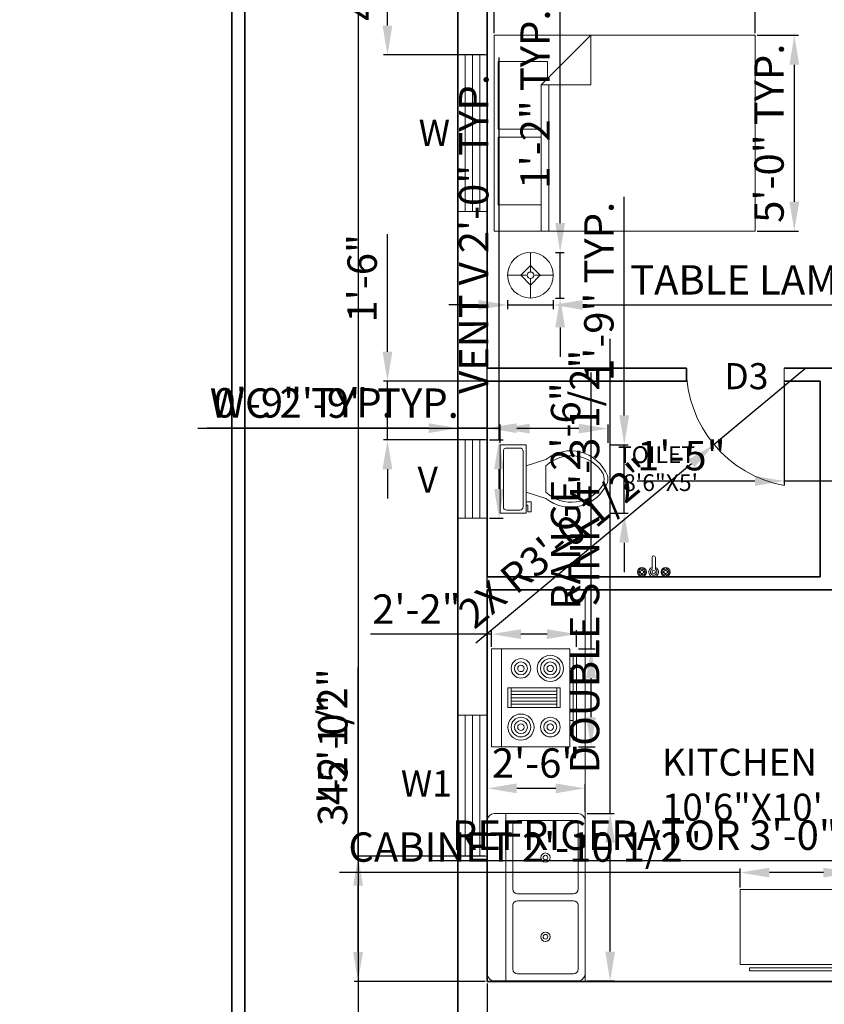
# Model space of a CAD drawing. Units: inches. Extents: x 2396 to 4051, y 1419 to 2191.
# Tile 2 of 7: x 2396 to 2642, y 1726 to 2028. Entities that reach past the tile are written whole.
import ezdxf

# ---------------------------------------------------------------- set-up
doc = ezdxf.new("R2010")
doc.units = ezdxf.units.IN
doc.layers.add('A-ANNO-TEXT', color=114, linetype='Continuous', lineweight=18, true_color=0x139b48)
doc.layers.add('A-GLAZ', color=52, linetype='Continuous', lineweight=18, true_color=0xc8c92d)
for name, color, linetype, lineweight in [('A-ANNO-TTLB', 7, 'Continuous', 35), ('A-AREA-IDEN', 6, 'Continuous', 18), ('A-DOOR', 4, 'Continuous', 18), ('A-EQPM', 8, 'Continuous', 18), ('A-FLOR-CASE', 9, 'Continuous', 18), ('A-FLOR-FIXT', 9, 'Continuous', 18), ('A-FURN', 8, 'Continuous', 18), ('A-WALL', 7, 'Continuous', 35), ('S-ANNO-DIMS', 2, 'Continuous', 18)]:
    doc.layers.add(name, color=color, linetype=linetype, lineweight=lineweight)
doc.styles.get("Standard").update_dxf_attribs({"font": 'arial.ttf'})
doc.dimstyles.new('ISO-25', dxfattribs={"dimtxt": 9, "dimasz": 9, "dimexe": 1.25, "dimexo": 0.625, "dimgap": 2, "dimtad": 1, "dimdec": 1, "dimlunit": 4, "dimtxsty": 'Standard', "dimcen": 2.5, "dimadec": 0, "dimazin": 0, "dimtfac": 1, "dimtdec": 1, "dimtmove": 0, "dimatfit": 3, "dimfxl": 1, "dimarcsym": 0})

# ---------------------------------------------------------------- blocks, each defined once
blk = doc.blocks.new('Wall Cabinet - 18 x 12 in side')
for points in [[(-12, -18), (-12, 0), (0, 0), (0, -18)], [(-13, -16.5), (-13, -1.5), (-12.5, -1.5), (-12.5, -16.5)]]:
    blk.add_lwpolyline(points, close=True)
blk = doc.blocks.new('Bed - Queen')
for p, q in [((0, -80.00003), (0, 0)), ((0, 0), (59.99999, 0)), ((59.99999, 0), (59.99999, -80.00003)), ((7.99999, -1.2), (28.79998, -1.2)), ((7.99999, -14.4), (7.99999, -1.2)), ((28.79998, -1.2), (28.79998, -14.4)), ((31.19999, -1.2), (51.99999, -1.2)), ((31.19999, -14.4), (31.19999, -1.2)), ((51.99999, -1.2), (51.99999, -16.4)), ((0, -14.4), (44.8, -14.4)), ((59.99999, -29.6), (44.8, -14.4)), ((44.8, -14.4), (44.8, -29.6)), ((44.8, -16.8), (0, -16.8)), ((51.99999, -16.4), (46.79936, -16.4)), ((44.8, -29.6), (59.99999, -29.6)), ((59.99999, -80.00003), (0, -80.00003))]:
    blk.add_line(p, q)
blk = doc.blocks.new('Lamp - Table')
for p, q in [((0, 7), (0, 1)), ((-1, 0), (-7, 0)), ((0, 3), (-3, 0)), ((-3, 0), (0, -3)), ((3, 0), (0, 3)), ((0, -3), (3, 0)), ((1, 0), (7, 0)), ((0, -1), (0, -7))]:
    blk.add_line(p, q)
for radius in [7, 1]:
    blk.add_circle((0, 0), radius)
blk = doc.blocks.new('Toilet - top')
for p, q in [((9.5, -6), (9.5, -2)), ((-10, -8.5), (-8, -8.5)), ((-10, -9.5), (-10, -8.5)), ((-8, -8.5), (-8, -8)), ((-7, -8), (-7, -9.5)), ((-4, -8), (-6, -14)), ((4, -8), (6, -14)), ((-7, -9.5), (-10, -9.5)), ((4, -14), (-4, -14))]:
    blk.add_line(p, q)
blk.add_lwpolyline([(10.5, -8), (10.5, 0), (-10.5, 0), (-10.5, -8)], close=True)
for points in [[(-9.5, -2), (-9.5, -6)], [(8.5, -1), (-8.5, -1)], [(-8.5, -7), (8.5, -7)]]:
    blk.add_lwpolyline(points)
for centre, radius, start, end in [((-8.62, -1.88), 0.884, 81.8699, 188.1301), ((8.62, -1.88), 0.884, 351.8699, 98.1301), ((-8.62, -6.12), 0.884, 171.8699, 278.1301), ((8.62, -6.12), 0.884, 261.8699, 8.1301), ((3.52, -21.58), 12.17, 141.4691, 247.9714), ((4.2, -21.82), 11.33, 136.3677, 238.9468), ((-3.52, -21.58), 12.17, 292.0284, 38.5307), ((-4.2, -21.82), 11.33, 301.053, 43.6321), ((0, -27.88), 4, 245.7318, 294.2682), ((0, -29), 4, 254.8605, 285.1395)]:
    blk.add_arc(centre, radius, start, end)
blk = doc.blocks.new('Faucet - Bathroom top')
for p, q in [((-4.107, 0.125), (-4.375, 0.125)), ((-3.75, 0.4788), (-3.75, 0.75)), ((-3.5, 0.482), (-3.5, 0.75)), ((-3.1461, 0.125), (-2.875, 0.125)), ((3.143, 0.125), (2.875, 0.125)), ((3.5, 0.4788), (3.5, 0.75)), ((3.75, 0.482), (3.75, 0.75)), ((4.1039, 0.125), (4.375, 0.125)), ((-4.1039, -0.125), (-4.375, -0.125)), ((-3.75, -0.4821), (-3.75, -0.75)), ((-3.5, -0.4789), (-3.5, -0.75)), ((-3.143, -0.125), (-2.875, -0.125)), ((-0.5, -0.8639), (-0.5, -4.5)), ((0.5, -4.5), (0.5, -0.8631)), ((3.1461, -0.125), (2.875, -0.125)), ((3.5, -0.4821), (3.5, -0.75)), ((3.75, -0.4789), (3.75, -0.75)), ((4.107, -0.125), (4.375, -0.125))]:
    blk.add_line(p, q)
for centre, radius in [((-3.625, 0), 1.375), ((-4.625, 0), 0.2795), ((-3.625, 0), 0.5), ((-3.625, 1), 0.2795), ((-2.625, 0), 0.2795), ((0, 0), 0.5), ((3.625, 0), 1.375), ((2.625, 0), 0.2795), ((3.625, 0), 0.5), ((3.625, 1), 0.2795), ((4.625, 0), 0.2795), ((-3.625, -1), 0.2795), ((3.625, -1), 0.2795)]:
    blk.add_circle(centre, radius)
for centre, radius, start, end in [((-3.625, 0), 1, 105.2407, 164.2093), ((-3.625, 0), 1, 16.44125, 74.07887), ((0, 0), 1.5, 289.6514, 250.3603), ((0, 0), 1, 300.3431, 239.7554), ((3.625, 0), 1, 106.12, 164.0884), ((3.625, 0), 1, 16.23422, 73.90469), ((-3.625, 0), 1, 196.2342, 253.9047), ((-3.625, 0), 1, 286.12, 344.0884), ((3.625, 0), 1, 196.4413, 254.0789), ((3.625, 0), 1, 285.2407, 344.2093), ((0, -4.5), 0.5, 180, 0)]:
    blk.add_arc(centre, radius, start, end)
blk = doc.blocks.new('Range-Oven - 30 in top')
for p, q in [((0, -3), (30, -3)), ((12, -6), (18, -6)), ((13, -20), (13, -6)), ((14, -6), (14, -20)), ((15, -20), (15, -6)), ((16, -6), (16, -20)), ((17, -20), (17, -6)), ((18, -20), (12, -20)), ((6, -24), (6, -25)), ((8, -25), (8, -24)), ((22, -25), (22, -24)), ((24, -24), (24, -25))]:
    blk.add_line(p, q)
for points in [[(0, -24), (0, 0), (30, 0), (30, -24)], [(12, -21), (12, -5), (18, -5), (18, -21)], [(2, -26), (2, -25), (28, -25), (28, -26)]]:
    blk.add_lwpolyline(points, close=True)
for centre, radius in [((6, -9), 4), ((6, -9), 3), ((24, -9), 3), ((6, -9), 2), ((6, -9), 1), ((24, -9), 2), ((24, -9), 1), ((6, -18), 3), ((24, -18), 4), ((24, -18), 3), ((6, -18), 2), ((6, -18), 1), ((24, -18), 2), ((24, -18), 1)]:
    blk.add_circle(centre, radius)
blk = doc.blocks.new('Sink-double - 36 in top')
for p, q in [((-18, -4), (18, -4)), ((-0.75, -18.5), (-0.75, -6.5)), ((0.75, -6.5), (0.75, -18.5))]:
    blk.add_line(p, q)
for points in [[(-16.5, 0), (16.5, 0)], [(-18, -19.5), (-18, -1.5)], [(18, -1.5), (18, -19.5)], [(-15.5, -5.5), (-1.75, -5.5)], [(1.75, -5.5), (15.5, -5.5)], [(-16.5, -18.5), (-16.5, -6.5)], [(16.5, -6.5), (16.5, -18.5)], [(16.5, -21), (-16.5, -21)], [(-1.75, -19.5), (-15.5, -19.5)], [(15.5, -19.5), (1.75, -19.5)]]:
    blk.add_lwpolyline(points)
for centre, radius in [((-8.5, -12.5), 1), ((-8.5, -12.5), 0.5), ((8.5, -12.5), 1), ((8.5, -12.5), 0.5)]:
    blk.add_circle(centre, radius)
for centre, radius, start, end in [((-16.5, -1.5), 1.5, 90, 180), ((16.5, -1.5), 1.5, 0, 90), ((-15.5, -6.5), 1, 90, 180), ((-1.75, -6.5), 1, 0, 90), ((1.75, -6.5), 1, 90, 180), ((15.5, -6.5), 1, 0, 90), ((-15.5, -18.5), 1, 180, 270), ((-1.75, -18.5), 1, 270, 0), ((1.75, -18.5), 1, 180, 270), ((15.5, -18.5), 1, 270, 0), ((-16.5, -19.5), 1.5, 180, 270), ((16.5, -19.5), 1.5, 270, 0)]:
    blk.add_arc(centre, radius, start, end)
blk = doc.blocks.new('WIN-W-48IN')
for p, q in [((0, 0), (0, 9)), ((0, 6.75), (48, 6.75)), ((48, 0), (48, 9)), ((0, 4.5), (48, 4.5)), ((0, 2.25), (48, 2.25))]:
    blk.add_line(p, q)
blk = doc.blocks.new('VENT-V-24IN')
for p, q in [((0, 0), (0, 9)), ((0, 6.75), (24, 6.75)), ((24, 0), (24, 9)), ((0, 4.5), (24, 4.5)), ((0, 2.25), (24, 2.25))]:
    blk.add_line(p, q)
blk = doc.blocks.new('WIN-W1-43P2IN')
for p, q in [((9, 43.2), (0, 43.2)), ((2.25, 0), (2.25, 43.2)), ((4.5, 0), (4.5, 43.2)), ((6.75, 0), (6.75, 43.2)), ((9, 0), (0, 0))]:
    blk.add_line(p, q)
blk = doc.blocks.new('DOOR-D3-36IN')
blk.add_line((30, 0), (30, 36))
blk.add_arc((36.6, 36), 36.6, 180, 259.6111)
blk = doc.blocks.new('*D40')
at = {"layer": 'Defpoints', "color": 0, "transparency": 16777216}
for p in [(2545.21, 1942.76), (2559.21, 1942.76), (2559.21, 1940.66)]:
    blk.add_point(p, dxfattribs=at)
at = {"layer": 'S-ANNO-DIMS', "color": 0, "lineweight": -2, "transparency": 16777216}
for p, q in [((2536.21, 1940.66), (2527.21, 1940.66)), ((2545.21, 1942.13), (2545.21, 1939.41)), ((2545.21, 1940.66), (2559.21, 1940.66)), ((2559.21, 1942.13), (2559.21, 1939.41)), ((2568.21, 1940.66), (2717.35, 1940.66))]:
    blk.add_line(p, q, dxfattribs=at)
at = {"layer": 'S-ANNO-DIMS', "color": 0, "transparency": 16777216}
for points in [[(2536.21, 1942.16), (2536.21, 1939.16), (2545.21, 1940.66)], [(2568.21, 1942.16), (2568.21, 1939.16), (2559.21, 1940.66)]]:
    blk.add_solid(points, dxfattribs=at)
at = {"layer": 'S-ANNO-DIMS', "color": 0, "transparency": 16777216, "insert": (2647.28, 1947.18), "char_height": 9, "attachment_point": 5}
blk.add_mtext('TABLE LAMP 1\'-2" TYP.', dxfattribs=at)
blk = doc.blocks.new('*D41')
at = {"layer": 'Defpoints', "color": 0, "transparency": 16777216}
for p in [(2559.21, 1956.76), (2561.31, 1956.76), (2559.21, 1942.76)]:
    blk.add_point(p, dxfattribs=at)
at = {"layer": 'S-ANNO-DIMS', "color": 0, "lineweight": -2, "transparency": 16777216}
for p, q in [((2561.31, 1965.76), (2561.31, 2032.77)), ((2559.83, 1956.76), (2562.56, 1956.76)), ((2561.31, 1942.76), (2561.31, 1956.76)), ((2559.83, 1942.76), (2562.56, 1942.76)), ((2561.31, 1933.76), (2561.31, 1924.76))]:
    blk.add_line(p, q, dxfattribs=at)
at = {"layer": 'S-ANNO-DIMS', "color": 0, "transparency": 16777216}
for points in [[(2559.81, 1965.76), (2562.81, 1965.76), (2561.31, 1956.76)], [(2559.81, 1933.76), (2562.81, 1933.76), (2561.31, 1942.76)]]:
    blk.add_solid(points, dxfattribs=at)
at = {"layer": 'S-ANNO-DIMS', "color": 0, "transparency": 16777216, "insert": (2554.79, 2003.76), "char_height": 9, "attachment_point": 5, "rotation": 90}
blk.add_mtext('1\'-2" TYP.', dxfattribs=at)
blk = doc.blocks.new('*D46')
at = {"layer": 'Defpoints', "color": 0, "transparency": 16777216}
for p in [(2541.07, 2035.3), (2541.07, 2023.3), (2621.07, 2023.3)]:
    blk.add_point(p, dxfattribs=at)
at = {"layer": 'S-ANNO-DIMS', "color": 0, "lineweight": -2, "transparency": 16777216}
for p, q in [((2541.07, 2035.3), (2395.68, 2035.3)), ((2541.07, 2023.93), (2541.07, 2036.55)), ((2612.07, 2035.3), (2550.07, 2035.3)), ((2621.07, 2023.93), (2621.07, 2036.55))]:
    blk.add_line(p, q, dxfattribs=at)
at = {"layer": 'S-ANNO-DIMS', "color": 0, "transparency": 16777216}
for points in [[(2550.07, 2036.8), (2550.07, 2033.8), (2541.07, 2035.3)], [(2612.07, 2036.8), (2612.07, 2033.8), (2621.07, 2035.3)]]:
    blk.add_solid(points, dxfattribs=at)
at = {"layer": 'S-ANNO-DIMS', "color": 0, "transparency": 16777216, "insert": (2463.87, 2042.23), "char_height": 9, "attachment_point": 5}
blk.add_mtext('QUEEN BED 6\'-8" TYP.', dxfattribs=at)
blk = doc.blocks.new('*D47')
at = {"layer": 'Defpoints', "color": 0, "transparency": 16777216}
for p in [(2621.07, 2023.3), (2633.07, 2023.3), (2621.07, 1963.3)]:
    blk.add_point(p, dxfattribs=at)
at = {"layer": 'S-ANNO-DIMS', "color": 0, "lineweight": -2, "transparency": 16777216}
for p, q in [((2621.7, 2023.3), (2634.32, 2023.3)), ((2633.07, 1972.3), (2633.07, 2014.3)), ((2621.7, 1963.3), (2634.32, 1963.3))]:
    blk.add_line(p, q, dxfattribs=at)
at = {"layer": 'S-ANNO-DIMS', "color": 0, "transparency": 16777216}
for points in [[(2631.57, 2014.3), (2634.57, 2014.3), (2633.07, 2023.3)], [(2631.57, 1972.3), (2634.57, 1972.3), (2633.07, 1963.3)]]:
    blk.add_solid(points, dxfattribs=at)
at = {"layer": 'S-ANNO-DIMS', "color": 0, "transparency": 16777216, "insert": (2626.48, 1993.3), "char_height": 9, "attachment_point": 5, "rotation": 90}
blk.add_mtext('5\'-0" TYP.', dxfattribs=at)
blk = doc.blocks.new('*D48')
at = {"layer": 'Defpoints', "color": 0, "transparency": 16777216}
for p in [(2542.93, 1902.76), (2542.93, 1897.8), (2575.98, 1897.8)]:
    blk.add_point(p, dxfattribs=at)
at = {"layer": 'S-ANNO-DIMS', "color": 0, "lineweight": -2, "transparency": 16777216}
for p, q in [((2542.93, 1902.76), (2450.26, 1902.76)), ((2542.93, 1898.43), (2542.93, 1904.01)), ((2566.98, 1902.76), (2551.93, 1902.76)), ((2575.98, 1898.43), (2575.98, 1904.01))]:
    blk.add_line(p, q, dxfattribs=at)
at = {"layer": 'S-ANNO-DIMS', "color": 0, "transparency": 16777216}
for points in [[(2551.93, 1904.26), (2551.93, 1901.26), (2542.93, 1902.76)], [(2566.98, 1904.26), (2566.98, 1901.26), (2575.98, 1902.76)]]:
    blk.add_solid(points, dxfattribs=at)
at = {"layer": 'S-ANNO-DIMS', "color": 0, "transparency": 16777216, "insert": (2492.1, 1909.41), "char_height": 9, "attachment_point": 5}
blk.add_mtext('WC 2\'-9" TYP.', dxfattribs=at)
blk = doc.blocks.new('*D49')
at = {"layer": 'Defpoints', "color": 0, "transparency": 16777216}
for p in [(2575.98, 1897.8), (2580.94, 1897.8), (2575.98, 1876.8)]:
    blk.add_point(p, dxfattribs=at)
at = {"layer": 'S-ANNO-DIMS', "color": 0, "lineweight": -2, "transparency": 16777216}
for p, q in [((2580.94, 1906.8), (2580.94, 1973.81)), ((2576.6, 1897.8), (2582.19, 1897.8)), ((2580.94, 1876.8), (2580.94, 1897.8)), ((2576.6, 1876.8), (2582.19, 1876.8)), ((2580.94, 1867.8), (2580.94, 1858.8))]:
    blk.add_line(p, q, dxfattribs=at)
at = {"layer": 'S-ANNO-DIMS', "color": 0, "transparency": 16777216}
for points in [[(2579.44, 1906.8), (2582.44, 1906.8), (2580.94, 1897.8)], [(2579.44, 1867.8), (2582.44, 1867.8), (2580.94, 1876.8)]]:
    blk.add_solid(points, dxfattribs=at)
at = {"layer": 'S-ANNO-DIMS', "color": 0, "transparency": 16777216, "insert": (2574.34, 1944.81), "char_height": 9, "attachment_point": 5, "rotation": 90}
blk.add_mtext('1\'-9" TYP.', dxfattribs=at)
blk = doc.blocks.new('*D52')
at = {"layer": 'Defpoints', "color": 0, "transparency": 16777216}
for p in [(2538.98, 1899.3), (2542.58, 1899.3), (2538.98, 1875.3)]:
    blk.add_point(p, dxfattribs=at)
at = {"layer": 'S-ANNO-DIMS', "color": 0, "lineweight": -2, "transparency": 16777216}
for p, q in [((2542.58, 1899.3), (2542.58, 2016.53)), ((2539.61, 1899.3), (2543.83, 1899.3)), ((2542.58, 1884.3), (2542.58, 1890.3)), ((2539.61, 1875.3), (2543.83, 1875.3))]:
    blk.add_line(p, q, dxfattribs=at)
at = {"layer": 'S-ANNO-DIMS', "color": 0, "transparency": 16777216}
for points in [[(2541.08, 1890.3), (2544.08, 1890.3), (2542.58, 1899.3)], [(2541.08, 1884.3), (2544.08, 1884.3), (2542.58, 1875.3)]]:
    blk.add_solid(points, dxfattribs=at)
at = {"layer": 'S-ANNO-DIMS', "color": 0, "transparency": 16777216, "insert": (2535.99, 1962.42), "char_height": 9, "attachment_point": 5, "rotation": 90}
blk.add_mtext('VENT V 2\'-0" TYP.', dxfattribs=at)
blk = doc.blocks.new('*D53')
at = {"layer": 'Defpoints', "color": 0, "transparency": 16777216}
for p in [(2529.98, 1902.9), (2529.98, 1899.3), (2538.98, 1899.3)]:
    blk.add_point(p, dxfattribs=at)
at = {"layer": 'S-ANNO-DIMS', "color": 0, "lineweight": -2, "transparency": 16777216}
for p, q in [((2520.98, 1902.9), (2453.12, 1902.9)), ((2529.98, 1899.93), (2529.98, 1904.15)), ((2538.98, 1902.9), (2529.98, 1902.9)), ((2538.98, 1899.93), (2538.98, 1904.15)), ((2547.98, 1902.9), (2556.98, 1902.9))]:
    blk.add_line(p, q, dxfattribs=at)
at = {"layer": 'S-ANNO-DIMS', "color": 0, "transparency": 16777216}
for points in [[(2520.98, 1904.4), (2520.98, 1901.4), (2529.98, 1902.9)], [(2547.98, 1904.4), (2547.98, 1901.4), (2538.98, 1902.9)]]:
    blk.add_solid(points, dxfattribs=at)
at = {"layer": 'S-ANNO-DIMS', "color": 0, "transparency": 16777216, "insert": (2482.55, 1909.5), "char_height": 9, "attachment_point": 5}
blk.add_mtext('0\'-9" TYP.', dxfattribs=at)
blk = doc.blocks.new('*D66')
at = {"layer": 'Defpoints', "color": 0, "transparency": 16777216}
for p in [(2661.68, 1770.32), (2661.68, 1764.92), (2697.68, 1764.92)]:
    blk.add_point(p, dxfattribs=at)
at = {"layer": 'S-ANNO-DIMS', "color": 0, "lineweight": -2, "transparency": 16777216}
for p, q in [((2661.68, 1765.55), (2661.68, 1771.57)), ((2697.68, 1765.55), (2697.68, 1771.57)), ((2661.68, 1770.32), (2521.84, 1770.32)), ((2688.68, 1770.32), (2670.68, 1770.32))]:
    blk.add_line(p, q, dxfattribs=at)
at = {"layer": 'S-ANNO-DIMS', "color": 0, "transparency": 16777216}
for points in [[(2670.68, 1771.82), (2670.68, 1768.82), (2661.68, 1770.32)], [(2688.68, 1771.82), (2688.68, 1768.82), (2697.68, 1770.32)]]:
    blk.add_solid(points, dxfattribs=at)
at = {"layer": 'S-ANNO-DIMS', "color": 0, "transparency": 16777216, "insert": (2587.26, 1776.98), "char_height": 9, "attachment_point": 5}
blk.add_mtext('REFRIGERATOR 3\'-0"', dxfattribs=at)
blk = doc.blocks.new('*D68')
at = {"layer": 'Defpoints', "color": 0, "transparency": 16777216}
for p in [(2616.45, 1766.68), (2616.45, 1761.5), (2650.99, 1761.5)]:
    blk.add_point(p, dxfattribs=at)
at = {"layer": 'S-ANNO-DIMS', "color": 0, "lineweight": -2, "transparency": 16777216}
for p, q in [((2616.45, 1766.68), (2493.68, 1766.68)), ((2616.45, 1762.12), (2616.45, 1767.93)), ((2641.99, 1766.68), (2625.45, 1766.68)), ((2650.99, 1762.12), (2650.99, 1767.93))]:
    blk.add_line(p, q, dxfattribs=at)
at = {"layer": 'S-ANNO-DIMS', "color": 0, "transparency": 16777216}
for points in [[(2625.45, 1768.18), (2625.45, 1765.18), (2616.45, 1766.68)], [(2641.99, 1768.18), (2641.99, 1765.18), (2650.99, 1766.68)]]:
    blk.add_solid(points, dxfattribs=at)
at = {"layer": 'S-ANNO-DIMS', "color": 0, "transparency": 16777216, "insert": (2550.56, 1773.33), "char_height": 9, "attachment_point": 5}
blk.add_mtext('CABINET 2\'-10 1/2"', dxfattribs=at)
blk = doc.blocks.new('*D72')
at = {"layer": 'Defpoints', "color": 0, "transparency": 16777216}
for p in [(2566.29, 1835.27), (2570.79, 1835.27), (2566.29, 1805.27)]:
    blk.add_point(p, dxfattribs=at)
at = {"layer": 'S-ANNO-DIMS', "color": 0, "lineweight": -2, "transparency": 16777216}
for p, q in [((2570.79, 1835.27), (2570.79, 1919.93)), ((2566.91, 1835.27), (2572.04, 1835.27)), ((2570.79, 1814.27), (2570.79, 1826.27)), ((2566.91, 1805.27), (2572.04, 1805.27))]:
    blk.add_line(p, q, dxfattribs=at)
at = {"layer": 'S-ANNO-DIMS', "color": 0, "transparency": 16777216}
for points in [[(2569.29, 1826.27), (2572.29, 1826.27), (2570.79, 1835.27)], [(2569.29, 1814.27), (2572.29, 1814.27), (2570.79, 1805.27)]]:
    blk.add_solid(points, dxfattribs=at)
at = {"layer": 'S-ANNO-DIMS', "color": 0, "transparency": 16777216, "insert": (2564.14, 1882.1), "char_height": 9, "attachment_point": 5, "rotation": 90}
blk.add_mtext('RANGE 2\'-6"', dxfattribs=at)
blk = doc.blocks.new('*D73')
at = {"layer": 'Defpoints', "color": 0, "transparency": 16777216}
for p in [(2540.29, 1839.77), (2540.29, 1835.27), (2566.29, 1835.27)]:
    blk.add_point(p, dxfattribs=at)
at = {"layer": 'S-ANNO-DIMS', "color": 0, "lineweight": -2, "transparency": 16777216}
for p, q in [((2540.29, 1835.89), (2540.29, 1841.02)), ((2566.29, 1835.89), (2566.29, 1841.02)), ((2540.29, 1839.77), (2503.21, 1839.77)), ((2557.29, 1839.77), (2549.29, 1839.77))]:
    blk.add_line(p, q, dxfattribs=at)
at = {"layer": 'S-ANNO-DIMS', "color": 0, "transparency": 16777216}
for points in [[(2549.29, 1841.27), (2549.29, 1838.27), (2540.29, 1839.77)], [(2557.29, 1841.27), (2557.29, 1838.27), (2566.29, 1839.77)]]:
    blk.add_solid(points, dxfattribs=at)
at = {"layer": 'S-ANNO-DIMS', "color": 0, "transparency": 16777216, "insert": (2517.25, 1846.29), "char_height": 9, "attachment_point": 5}
blk.add_mtext('2\'-2"', dxfattribs=at)
blk = doc.blocks.new('*D74')
at = {"layer": 'Defpoints', "color": 0, "transparency": 16777216}
for p in [(2568.93, 1784.8), (2576.63, 1784.8), (2568.93, 1733.47)]:
    blk.add_point(p, dxfattribs=at)
at = {"layer": 'S-ANNO-DIMS', "color": 0, "lineweight": -2, "transparency": 16777216}
for p, q in [((2576.63, 1784.8), (2576.63, 1930.28)), ((2569.55, 1784.8), (2577.88, 1784.8)), ((2576.63, 1742.47), (2576.63, 1775.8)), ((2569.55, 1733.47), (2577.88, 1733.47))]:
    blk.add_line(p, q, dxfattribs=at)
at = {"layer": 'S-ANNO-DIMS', "color": 0, "transparency": 16777216}
for points in [[(2575.13, 1775.8), (2578.13, 1775.8), (2576.63, 1784.8)], [(2575.13, 1742.47), (2578.13, 1742.47), (2576.63, 1733.47)]]:
    blk.add_solid(points, dxfattribs=at)
at = {"layer": 'S-ANNO-DIMS', "color": 0, "transparency": 16777216, "insert": (2569.97, 1862.04), "char_height": 9, "attachment_point": 5, "rotation": 90}
blk.add_mtext('DOUBLE SINK 4\'-3 1/2"', dxfattribs=at)
blk = doc.blocks.new('*D75')
at = {"layer": 'Defpoints', "color": 0, "transparency": 16777216}
for p in [(2538.98, 1792.5), (2538.98, 1784.8), (2568.93, 1784.8)]:
    blk.add_point(p, dxfattribs=at)
at = {"layer": 'S-ANNO-DIMS', "color": 0, "lineweight": -2, "transparency": 16777216}
for p, q in [((2538.98, 1785.43), (2538.98, 1793.75)), ((2568.93, 1785.43), (2568.93, 1793.75)), ((2559.93, 1792.5), (2547.98, 1792.5))]:
    blk.add_line(p, q, dxfattribs=at)
at = {"layer": 'S-ANNO-DIMS', "color": 0, "transparency": 16777216}
for points in [[(2547.98, 1794), (2547.98, 1791), (2538.98, 1792.5)], [(2559.93, 1794), (2559.93, 1791), (2568.93, 1792.5)]]:
    blk.add_solid(points, dxfattribs=at)
at = {"layer": 'S-ANNO-DIMS', "color": 0, "transparency": 16777216, "insert": (2553.95, 1799.1), "char_height": 9, "attachment_point": 5}
blk.add_mtext('2\'-6"', dxfattribs=at)
blk = doc.blocks.new('*D77')
at = {"layer": 'Defpoints', "color": 0, "transparency": 16777216}
for p in [(2529.98, 2074.3), (2499.38, 1534.3), (2774.98, 1534.3)]:
    blk.add_point(p, dxfattribs=at)
at = {"layer": 'S-ANNO-DIMS', "color": 0, "lineweight": -2, "transparency": 16777216}
for p, q in [((2529.36, 2074.3), (2498.13, 2074.3)), ((2499.38, 2065.3), (2499.38, 1543.3)), ((2774.36, 1534.3), (2498.13, 1534.3))]:
    blk.add_line(p, q, dxfattribs=at)
at = {"layer": 'S-ANNO-DIMS', "color": 0, "transparency": 16777216}
for points in [[(2497.88, 2065.3), (2500.88, 2065.3), (2499.38, 2074.3)], [(2497.88, 1543.3), (2500.88, 1543.3), (2499.38, 1534.3)]]:
    blk.add_solid(points, dxfattribs=at)
at = {"layer": 'S-ANNO-DIMS', "color": 0, "transparency": 16777216, "insert": (2492.79, 1804.3), "char_height": 9, "attachment_point": 5, "rotation": 90}
blk.add_mtext('45\'-0"', dxfattribs=at)
blk = doc.blocks.new('*D78')
at = {"layer": 'Defpoints', "color": 0, "transparency": 16777216}
for p in [(2538.98, 1733.3), (2706.98, 1733.3), (2706.98, 1503.7)]:
    blk.add_point(p, dxfattribs=at)
at = {"layer": 'S-ANNO-DIMS', "color": 0, "lineweight": -2, "transparency": 16777216}
for p, q in [((2538.98, 1732.68), (2538.98, 1502.45)), ((2706.98, 1732.68), (2706.98, 1502.45)), ((2547.98, 1503.7), (2697.98, 1503.7))]:
    blk.add_line(p, q, dxfattribs=at)
at = {"layer": 'S-ANNO-DIMS', "color": 0, "transparency": 16777216}
for points in [[(2547.98, 1505.2), (2547.98, 1502.2), (2538.98, 1503.7)], [(2697.98, 1505.2), (2697.98, 1502.2), (2706.98, 1503.7)]]:
    blk.add_solid(points, dxfattribs=at)
at = {"layer": 'S-ANNO-DIMS', "color": 0, "transparency": 16777216, "insert": (2622.98, 1510.3), "char_height": 9, "attachment_point": 5}
blk.add_mtext('14\'-0"', dxfattribs=at)
blk = doc.blocks.new('*D89')
at = {"layer": 'Defpoints', "color": 0, "transparency": 16777216}
for p in [(2499.38, 1771.7), (2538.98, 1771.7), (2538.98, 1733.3)]:
    blk.add_point(p, dxfattribs=at)
at = {"layer": 'S-ANNO-DIMS', "color": 0, "lineweight": -2, "transparency": 16777216}
for p, q in [((2499.38, 1771.7), (2499.38, 1829.59)), ((2538.36, 1771.7), (2498.13, 1771.7)), ((2499.38, 1742.3), (2499.38, 1762.7)), ((2538.36, 1733.3), (2498.13, 1733.3))]:
    blk.add_line(p, q, dxfattribs=at)
at = {"layer": 'S-ANNO-DIMS', "color": 0, "transparency": 16777216}
for points in [[(2497.88, 1762.7), (2500.88, 1762.7), (2499.38, 1771.7)], [(2497.88, 1742.3), (2500.88, 1742.3), (2499.38, 1733.3)]]:
    blk.add_solid(points, dxfattribs=at)
at = {"layer": 'S-ANNO-DIMS', "color": 0, "transparency": 16777216, "insert": (2492.73, 1805.15), "char_height": 9, "attachment_point": 5, "rotation": 90}
blk.add_mtext('3\'-2 1/2"', dxfattribs=at)
blk = doc.blocks.new('*D91')
at = {"layer": 'Defpoints', "color": 0, "transparency": 16777216}
for p in [(2508.38, 2065.3), (2538.98, 2065.3), (2538.98, 2017.3)]:
    blk.add_point(p, dxfattribs=at)
at = {"layer": 'S-ANNO-DIMS', "color": 0, "lineweight": -2, "transparency": 16777216}
for p, q in [((2538.36, 2065.3), (2507.13, 2065.3)), ((2508.38, 2026.3), (2508.38, 2056.3)), ((2538.36, 2017.3), (2507.13, 2017.3))]:
    blk.add_line(p, q, dxfattribs=at)
at = {"layer": 'S-ANNO-DIMS', "color": 0, "transparency": 16777216}
for points in [[(2506.88, 2056.3), (2509.88, 2056.3), (2508.38, 2065.3)], [(2506.88, 2026.3), (2509.88, 2026.3), (2508.38, 2017.3)]]:
    blk.add_solid(points, dxfattribs=at)
at = {"layer": 'S-ANNO-DIMS', "color": 0, "transparency": 16777216, "insert": (2501.79, 2041.3), "char_height": 9, "attachment_point": 5, "rotation": 90}
blk.add_mtext('4\'-0"', dxfattribs=at)
blk = doc.blocks.new('*D92')
at = {"layer": 'Defpoints', "color": 0, "transparency": 16777216}
for p in [(2508.38, 1917.3), (2538.98, 1917.3), (2538.98, 1899.3)]:
    blk.add_point(p, dxfattribs=at)
at = {"layer": 'S-ANNO-DIMS', "color": 0, "lineweight": -2, "transparency": 16777216}
for p, q in [((2508.38, 1926.3), (2508.38, 1962.38)), ((2538.36, 1917.3), (2507.13, 1917.3)), ((2508.38, 1899.3), (2508.38, 1917.3)), ((2538.36, 1899.3), (2507.13, 1899.3)), ((2508.38, 1890.3), (2508.38, 1881.3))]:
    blk.add_line(p, q, dxfattribs=at)
at = {"layer": 'S-ANNO-DIMS', "color": 0, "transparency": 16777216}
for points in [[(2506.88, 1926.3), (2509.88, 1926.3), (2508.38, 1917.3)], [(2506.88, 1890.3), (2509.88, 1890.3), (2508.38, 1899.3)]]:
    blk.add_solid(points, dxfattribs=at)
at = {"layer": 'S-ANNO-DIMS', "color": 0, "transparency": 16777216, "insert": (2501.79, 1948.84), "char_height": 9, "attachment_point": 5, "rotation": 90}
blk.add_mtext('1\'-6"', dxfattribs=at)
blk = doc.blocks.new('*D95')
at = {"layer": 'Defpoints', "color": 0, "transparency": 16777216}
for p in [(2646.98, 2154.77), (2538.98, 1853.3), (2646.98, 1853.3)]:
    blk.add_point(p, dxfattribs=at)
at = {"layer": 'S-ANNO-DIMS', "color": 0, "lineweight": -2, "transparency": 16777216}
for p, q in [((2538.98, 1853.93), (2538.98, 2156.02)), ((2547.98, 2154.77), (2637.98, 2154.77)), ((2646.98, 1853.93), (2646.98, 2156.02))]:
    blk.add_line(p, q, dxfattribs=at)
at = {"layer": 'S-ANNO-DIMS', "color": 0, "transparency": 16777216}
for points in [[(2547.98, 2156.27), (2547.98, 2153.27), (2538.98, 2154.77)], [(2637.98, 2156.27), (2637.98, 2153.27), (2646.98, 2154.77)]]:
    blk.add_solid(points, dxfattribs=at)
at = {"layer": 'S-ANNO-DIMS', "color": 0, "transparency": 16777216, "insert": (2592.98, 2161.37), "char_height": 9, "attachment_point": 5}
blk.add_mtext('9\'-0"', dxfattribs=at)
blk = doc.blocks.new('*D98')
at = {"layer": 'Defpoints', "color": 0, "transparency": 16777216}
for p in [(2629.98, 1917.3), (2646.98, 1917.3), (2629.98, 1886.7)]:
    blk.add_point(p, dxfattribs=at)
at = {"layer": 'S-ANNO-DIMS', "color": 0, "lineweight": -2, "transparency": 16777216}
for p, q in [((2629.98, 1916.68), (2629.98, 1885.45)), ((2646.98, 1916.68), (2646.98, 1885.45)), ((2620.98, 1886.7), (2584.91, 1886.7)), ((2646.98, 1886.7), (2629.98, 1886.7)), ((2655.98, 1886.7), (2664.98, 1886.7))]:
    blk.add_line(p, q, dxfattribs=at)
at = {"layer": 'S-ANNO-DIMS', "color": 0, "transparency": 16777216}
for points in [[(2620.98, 1888.2), (2620.98, 1885.2), (2629.98, 1886.7)], [(2655.98, 1888.2), (2655.98, 1885.2), (2646.98, 1886.7)]]:
    blk.add_solid(points, dxfattribs=at)
at = {"layer": 'S-ANNO-DIMS', "color": 0, "transparency": 16777216, "insert": (2598.45, 1893.3), "char_height": 9, "attachment_point": 5}
blk.add_mtext('1\'-5"', dxfattribs=at)
blk = doc.blocks.new('*D115')
at = {"layer": 'Defpoints', "color": 0, "transparency": 16777216}
for p in [(2636.58, 1921.3), (2608.47, 1897.87)]:
    blk.add_point(p, dxfattribs=at)
at = {"layer": 'S-ANNO-DIMS', "color": 0, "lineweight": -2, "transparency": 16777216}
for p, q in [((2636.58, 1921.3), (2608.47, 1897.87)), ((2535.49, 1837.05), (2601.55, 1892.11))]:
    blk.add_line(p, q, dxfattribs=at)
at = {"layer": 'S-ANNO-DIMS', "color": 0, "transparency": 16777216}
blk.add_solid([(2600.59, 1893.26), (2602.51, 1890.96), (2608.47, 1897.87)], dxfattribs=at)
at = {"layer": 'S-ANNO-DIMS', "color": 0, "transparency": 16777216, "insert": (2560.8, 1866.81), "char_height": 9, "attachment_point": 5, "rotation": 39.8055}
blk.add_mtext('2X R3\'-0 1/2"', dxfattribs=at)

msp = doc.modelspace()

# ---------------------------------------------------------------- linework, layer by layer
at = {"layer": 'A-ANNO-TTLB'}
for points in [[(2460.66, 2191.26), (4051.21, 2191.26), (4051.21, 1469.82), (2460.66, 1469.82)], [(2464.66, 2187.26), (4047.21, 2187.26), (4047.21, 1473.82), (2464.66, 1473.82)]]:
    msp.add_lwpolyline(points, close=True, dxfattribs=at)
at = {"layer": 'A-FLOR-CASE'}
msp.add_line((2568.98, 1733.3), (2568.98, 1853.3), dxfattribs=at)
at = {"layer": 'A-WALL'}
for p, q in [((2529.98, 1632.3), (2529.98, 2074.3)), ((2538.98, 1921.3), (2538.98, 2065.3)), ((2599.98, 1921.3), (2538.98, 1921.3)), ((2599.98, 1917.3), (2599.98, 1921.3)), ((2646.98, 1921.3), (2629.98, 1921.3)), ((2538.98, 1857.3), (2538.98, 1917.3)), ((2599.98, 1917.3), (2538.98, 1917.3)), ((2640.98, 1917.3), (2629.98, 1917.3)), ((2640.98, 1857.3), (2640.98, 1917.3)), ((2640.98, 1857.3), (2538.98, 1857.3)), ((2538.98, 1733.3), (2538.98, 1853.3)), ((2644.98, 1853.3), (2538.98, 1853.3)), ((2706.98, 1733.3), (2538.98, 1733.3))]:
    msp.add_line(p, q, dxfattribs=at)

# ---------------------------------------------------------------- block references
at = {"layer": 'A-DOOR'}
msp.add_blockref('DOOR-D3-36IN', (2599.98, 1885.3), dxfattribs=at)
at = {"layer": 'A-EQPM', "rotation": 90}
msp.add_blockref('Range-Oven - 30 in top', (2540.29, 1805.27), dxfattribs=at)
at = {"layer": 'A-FLOR-CASE', "xscale": 1.91927912988188, "yscale": 1.91927912988188, "zscale": 1.91927912988188, "rotation": 90}
msp.add_blockref('Wall Cabinet - 18 x 12 in side', (2616.45, 1761.5), dxfattribs=at)
at = {"layer": 'A-FLOR-FIXT'}
for name, p, rotation in [('Toilet - top', (2542.93, 1887.3), 90), ('Faucet - Bathroom top', (2589.98, 1858.8), 180)]:
    msp.add_blockref(name, p, dxfattribs=dict(at, rotation=rotation))
at = {"layer": 'A-FLOR-FIXT', "xscale": 1.425817307797755, "yscale": 1.425817307797755, "zscale": 1.425817307797755, "rotation": 90}
msp.add_blockref('Sink-double - 36 in top', (2538.98, 1759.14), dxfattribs=at)
at = {"layer": 'A-FURN', "rotation": 90}
msp.add_blockref('Bed - Queen', (2541.07, 1963.3), dxfattribs=at)
at = {"layer": 'A-FURN'}
msp.add_blockref('Lamp - Table', (2552.21, 1949.76), dxfattribs=at)
at = {"layer": 'A-GLAZ'}
for name, p, rotation in [('WIN-W-48IN', (2538.98, 1969.3), 89.99999999999905), ('VENT-V-24IN', (2538.98, 1875.3), 89.99999999999895)]:
    msp.add_blockref(name, p, dxfattribs=dict(at, rotation=rotation))
msp.add_blockref('WIN-W1-43P2IN', (2529.98, 1771.7), dxfattribs=at)

# ---------------------------------------------------------------- texts
at = {"layer": 'A-ANNO-TEXT', "char_height": 8, "attachment_point": 1}
for s, insert in [('W', (2517.96, 1997.42)), ('{D3}', (2611.59, 1922.83)), ('V', (2517.58, 1891.13)), ('W1', (2512.5, 1797.99))]:
    msp.add_mtext_dynamic_manual_height_columns(s, width=139.3028, gutter_width=12.5, heights=[0], dxfattribs=dict(at, insert=insert))
at = {"layer": 'A-AREA-IDEN', "attachment_point": 1}
for s, width, gutter_width, insert, char_height in [('   TOILET\\P    8\'6"X5\'', 89.5376, 8.03, (2574.33, 1897.34), 5.142), ('   KITCHEN\\P   10\'6"X10\'', 143.7762, 12.9, (2584.92, 1804.62), 8.2569)]:
    msp.add_mtext_dynamic_manual_height_columns(s, width=width, gutter_width=gutter_width, heights=[0], dxfattribs=dict(at, insert=insert, char_height=char_height))

# ---------------------------------------------------------------- dimensions: what is measured, and where the dimension line sits
at = {"layer": 'S-ANNO-DIMS'}
for base, p1, p2, picture, middle in [((2646.98, 2154.77), (2538.98, 1853.3), (2646.98, 1853.3), '*D95', (2592.98, 2161.37)), ((2706.98, 1503.7), (2538.98, 1733.3), (2706.98, 1733.3), '*D78', (2622.98, 1510.3))]:
    dim = msp.add_linear_dim(base=base, p1=p1, p2=p2, dimstyle='ISO-25', override={"dimdec": 1, "dimlfac": 1, "dimrnd": 0, "dimzin": 1, "dimdsep": 46, "dimlunit": 4, "dimfrac": 2}, dxfattribs=at)
    dim.commit()
    dim.dimension.update_dxf_attribs({"geometry": picture, "text_midpoint": middle})
for base, p1, p2, angle, picture, middle in [((2499.38, 1534.3), (2529.98, 2074.3), (2774.98, 1534.3), 90, '*D77', (2492.79, 1804.3)), ((2508.38, 2065.3), (2538.98, 2017.3), (2538.98, 2065.3), 90, '*D91', (2501.79, 2041.3)), ((2508.38, 1917.3), (2538.98, 1899.3), (2538.98, 1917.3), 90, '*D92', (2501.79, 1948.84)), ((2629.98, 1886.7), (2646.98, 1917.3), (2629.98, 1917.3), 180, '*D98', (2598.45, 1893.3)), ((2540.29, 1839.77), (2566.29, 1835.27), (2540.29, 1835.27), 180, '*D73', (2517.25, 1846.29)), ((2499.38, 1771.7), (2538.98, 1733.3), (2538.98, 1771.7), 90, '*D89', (2492.73, 1805.15)), ((2538.9839, 1792.5014), (2568.926, 1784.802), (2538.9839, 1784.802), 180, '*D75', (2553.955, 1799.0965))]:
    dim = msp.add_linear_dim(base=base, p1=p1, p2=p2, angle=angle, dimstyle='ISO-25', override={"dimdec": 1, "dimlfac": 1, "dimrnd": 0, "dimzin": 1, "dimdsep": 46, "dimlunit": 4, "dimfrac": 2}, dxfattribs=at)
    dim.commit()
    dim.dimension.update_dxf_attribs({"geometry": picture, "text_midpoint": middle})
for base, p1, p2, angle, text, picture, middle in [((2541.07, 2035.3), (2621.07, 2023.3), (2541.07, 2023.3), 180, 'QUEEN BED <> TYP.', '*D46', (2463.87, 2042.23)), ((2561.31, 1956.76), (2559.21, 1942.76), (2559.21, 1956.76), 90, '<> TYP.', '*D41', (2554.79, 2003.76)), ((2633.07, 2023.3), (2621.07, 1963.3), (2621.07, 2023.3), 90, '<> TYP.', '*D47', (2626.48, 1993.3)), ((2542.58, 1899.3), (2538.98, 1875.3), (2538.98, 1899.3), 90, 'VENT V <> TYP.', '*D52', (2535.99, 1962.42)), ((2580.94, 1897.8), (2575.98, 1876.8), (2575.98, 1897.8), 90, '<> TYP.', '*D49', (2574.34, 1944.81)), ((2542.9323, 1902.7576), (2575.9785, 1897.8006), (2542.9323, 1897.8006), 180, 'WC <> TYP.', '*D48', (2492.0984, 1909.4111)), ((2576.63, 1784.8), (2568.93, 1733.47), (2568.93, 1784.8), 90, 'DOUBLE SINK <>', '*D74', (2569.97, 1862.04)), ((2529.98, 1902.9), (2538.98, 1899.3), (2529.98, 1899.3), 180, '<> TYP.', '*D53', (2482.55, 1909.5)), ((2570.79, 1835.27), (2566.29, 1805.27), (2566.29, 1835.27), 90, 'RANGE <>', '*D72', (2564.14, 1882.1)), ((2616.45, 1766.68), (2650.99, 1761.5), (2616.45, 1761.5), 180, 'CABINET <>', '*D68', (2550.56, 1773.33)), ((2661.68, 1770.32), (2697.68, 1764.92), (2661.68, 1764.92), 180, 'REFRIGERATOR <>', '*D66', (2587.26, 1776.98))]:
    dim = msp.add_linear_dim(base=base, p1=p1, p2=p2, angle=angle, text=text, dimstyle='ISO-25', override={"dimdec": 1, "dimlfac": 1, "dimrnd": 0, "dimzin": 1, "dimdsep": 46, "dimlunit": 4, "dimfrac": 2}, dxfattribs=at)
    dim.commit()
    dim.dimension.update_dxf_attribs({"geometry": picture, "text_midpoint": middle})
dim = msp.add_linear_dim(base=(2559.21, 1940.66), p1=(2545.21, 1942.76), p2=(2559.21, 1942.76), text='TABLE LAMP <> TYP.', dimstyle='ISO-25', override={"dimdec": 1, "dimlfac": 1, "dimrnd": 0, "dimzin": 1, "dimdsep": 46, "dimlunit": 4, "dimfrac": 2}, dxfattribs=at)
dim.commit()
dim.dimension.update_dxf_attribs({"geometry": '*D40', "text_midpoint": (2647.28, 1947.18)})
dim = msp.add_radius_dim(center=(2636.58, 1921.3), mpoint=(2608.47, 1897.87), text='2X <>', dimstyle='ISO-25', override={"dimdec": 1, "dimlfac": 1, "dimrnd": 0, "dimzin": 1, "dimdsep": 46, "dimlunit": 4, "dimfrac": 2}, dxfattribs=at)
dim.commit()
dim.dimension.update_dxf_attribs({"geometry": '*D115', "text_midpoint": (2560.8, 1866.81)})

doc.saveas('drawing.dxf')
